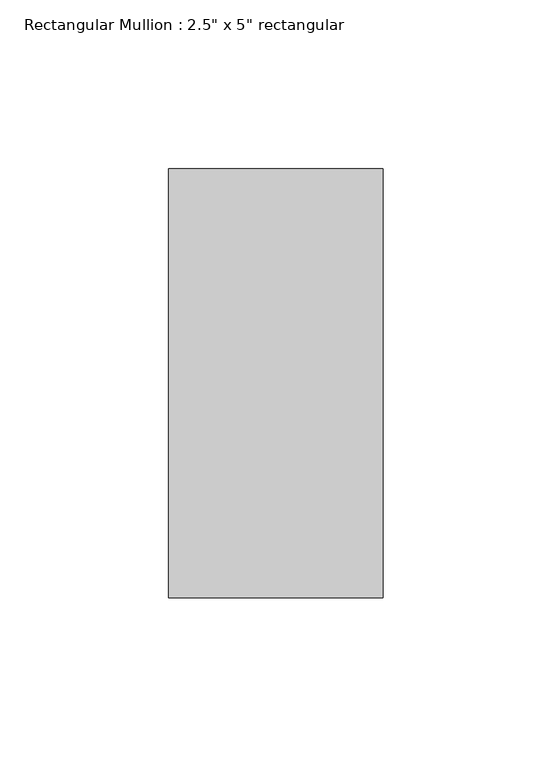
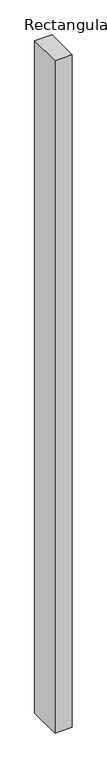
"""IFC4 building model written with IfcOpenShell, lengths in millimetres: member geometry."""

from ifc_helpers import new_model, si_unit, frame, origin, place, context, project, spatial, polyline, outline, extrude, source, transform, mapped, element, save


def member_9f3fc137(model_context):
    return source(origin(), model_context, "Body", "SweptSolid", [
        extrude(outline(polyline([(0.0, 63.5), (0.0, -63.5), (-63.5, -63.5), (-63.5, 63.5), (0.0, 63.5)])), frame((0.0, 0.0, -2590.8), z_axis=(0.0, 0.0, 1.0), x_axis=(1.0, 0.0, 0.0)), (0.0, 0.0, 1.0), 2590.8),
    ])


if __name__ == "__main__":
    model = new_model("IFC4")
    model_context = context("Model", 3, world=origin())
    ifc_project = project(units=[si_unit("LENGTHUNIT", "METRE", prefix="MILLI")], contexts=[model_context])
    site = spatial("IfcSite", under=ifc_project)
    building = spatial("IfcBuilding", under=site)
    placement = place(None, origin())
    member_shape = member_9f3fc137(model_context)
    element("IfcMember", 1, ObjectType="Rectangular Mullion : 2.5\" x 5\" rectangular", at=placement, inside=building, context=model_context, shape_type="MappedRepresentation", body=[
        mapped(member_shape, transform((0.0, 0.0, 0.0), x_axis=(1.0, 0.0, 0.0), y_axis=(0.0, 1.0, 0.0), z_axis=(0.0, 0.0, 1.0))),
    ])
    save(model, "model.ifc")

# Revit data of these elements
# Type "Rectangular Mullion : 2.5\" x 5\" rectangular"
#   built-in parameter 1007304 = 0.416667 (stored number, unit not read)
#   built-in parameter 1007301 = 0.104167 (stored number, unit not read)
#   built-in parameter 1007300 = 0.104167 (stored number, unit not read)
# Element 1 (IfcMember, "Rectangular Mullion : 2.5\" x 5\" rectangular")
#   Materials on its faces: "WINDOW FRAMING"
# Materials
#   "WINDOW FRAMING": class "Generic", colour RGB 120 120 120, transparency 0, Cost = 0
